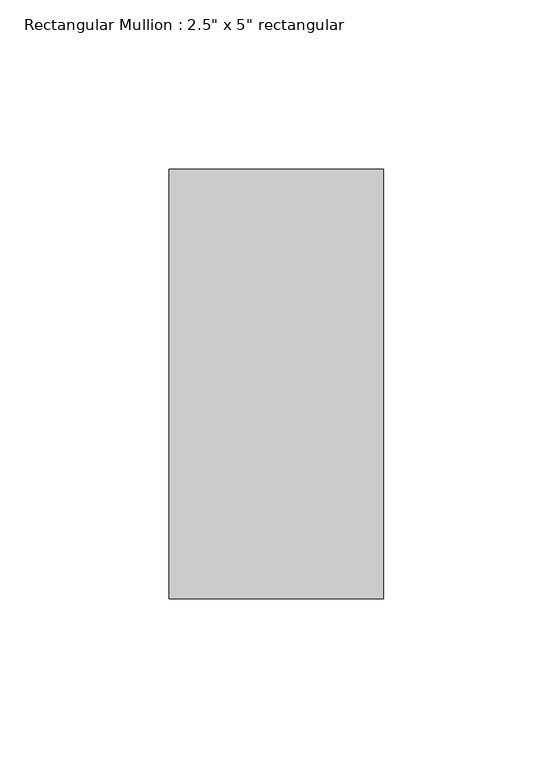
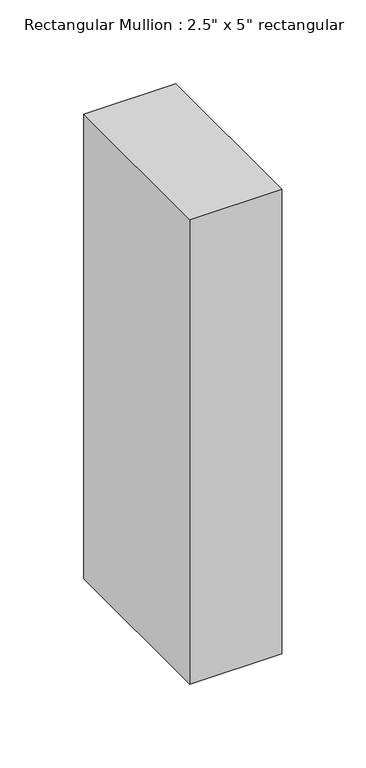
"""IFC4 building model written with IfcOpenShell, lengths in millimetres: member geometry."""

from ifc_helpers import new_model, si_unit, frame, origin, place, context, project, spatial, polyline, outline, extrude, source, transform, mapped, element, save


def member_d39130fe(model_context):
    return source(origin(), model_context, "Body", "SweptSolid", [
        extrude(outline(polyline([(0.0, 63.5), (0.0, -63.5), (-63.5, -63.5), (-63.5, 63.5), (0.0, 63.5)])), frame((0.0, 0.0, -338.9748327), z_axis=(0.0, 0.0, 1.0), x_axis=(1.0, 0.0, 0.0)), (0.0, 0.0, 1.0), 338.9748327),
    ])


if __name__ == "__main__":
    model = new_model("IFC4")
    model_context = context("Model", 3, world=origin())
    ifc_project = project(units=[si_unit("LENGTHUNIT", "METRE", prefix="MILLI")], contexts=[model_context])
    site = spatial("IfcSite", under=ifc_project)
    building = spatial("IfcBuilding", under=site)
    placement = place(None, origin())
    member_shape = member_d39130fe(model_context)
    element("IfcMember", 1, ObjectType="Rectangular Mullion : 2.5\" x 5\" rectangular", at=placement, inside=building, context=model_context, shape_type="MappedRepresentation", body=[
        mapped(member_shape, transform((0.0, 0.0, 0.0), x_axis=(1.0, 0.0, 0.0), y_axis=(0.0, 1.0, 0.0), z_axis=(0.0, 0.0, 1.0))),
    ])
    save(model, "model.ifc")

# Revit data of these elements
# Type "Rectangular Mullion : 2.5\" x 5\" rectangular"
#   built-in parameter 1007304 = 0.416667 (stored number, unit not read)
#   built-in parameter 1007301 = 0.104167 (stored number, unit not read)
#   built-in parameter 1007300 = 0.104167 (stored number, unit not read)
# Element 1 (IfcMember, "Rectangular Mullion : 2.5\" x 5\" rectangular")
#   Materials on its faces: "Aluminum"
# Materials
#   "Aluminum": class "Metal", colour RGB 247 247 247, transparency 0, Description = "Aluminum 6061", Cost = 0
